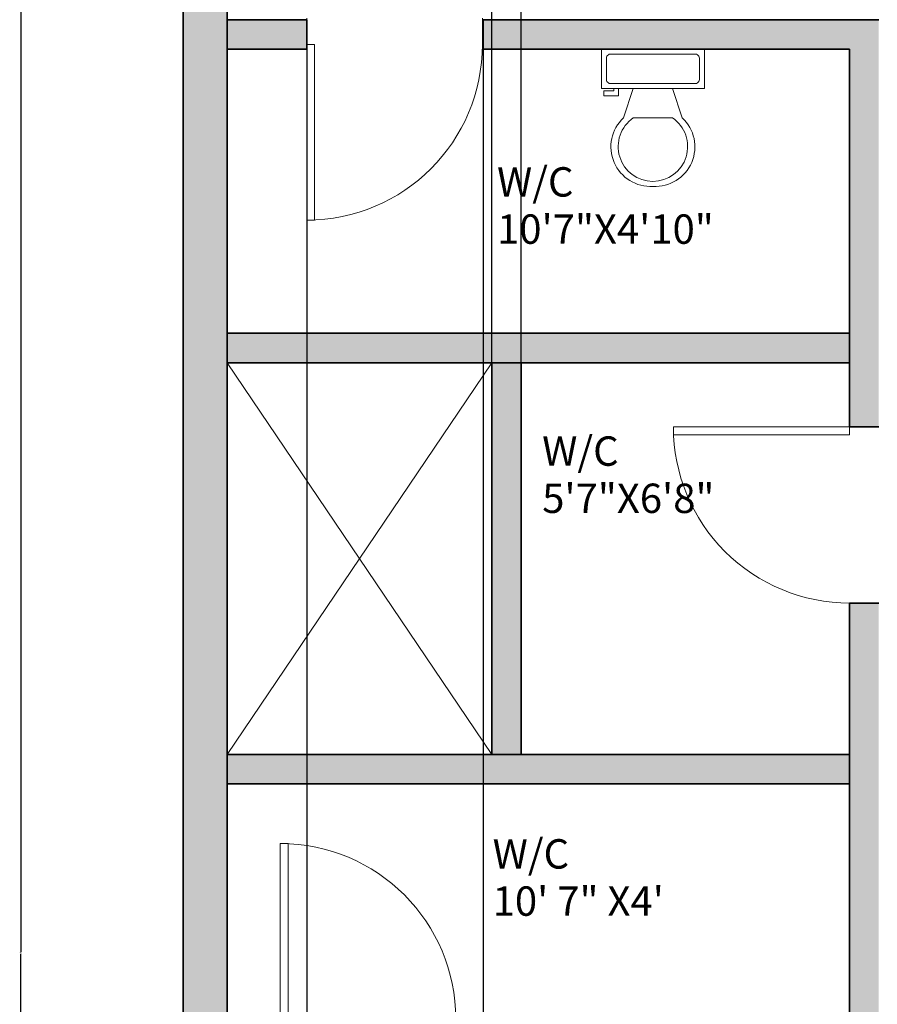
# Model space of a CAD drawing. Units: inches. Extents: x 2070 to 4408, y 1595 to 4269.
# Tile 9 of 20: x 2070 to 2245, y 1949 to 2150. Entities that reach past the tile are written whole.
import ezdxf

# ---------------------------------------------------------------- set-up
doc = ezdxf.new("R2010")
doc.units = ezdxf.units.IN
for name, color, linetype, lineweight in [('A-ANNO-DIMS', 2, 'Continuous', 18), ('A-AREA-IDEN', 7, 'Continuous', 18), ('A-DOOR', 4, 'Continuous', 18), ('A-FLOR-FIXT', 9, 'Continuous', 18), ('A-FLOR-OPEN', 8, 'Continuous', 13), ('A-WALL', 7, 'Continuous', 35)]:
    doc.layers.add(name, color=color, linetype=linetype, lineweight=lineweight)
doc.layers.add('A-WALL-PATT', color=18, linetype='Continuous', lineweight=13, true_color=0x000000)
doc.styles.get("Standard").update_dxf_attribs({"font": 'arial.ttf'})
doc.dimstyles.get("Standard").update_dxf_attribs({"dimtxt": 0.18, "dimasz": 0.18, "dimexe": 0.18, "dimexo": 0.0625, "dimgap": 0.09, "dimtad": 0, "dimtih": 1, "dimtoh": 1, "dimdec": 4, "dimzin": 0, "dimdsep": 46, "dimtxsty": 'Standard', "dimcen": 0.09, "dimadec": 0, "dimazin": 0, "dimtfac": 1, "dimtdec": 4, "dimtofl": 0, "dimtmove": 0, "dimatfit": 3, "dimfxl": 1, "dimtolj": 1, "dimtzin": 0, "dimarcsym": 0})

# ---------------------------------------------------------------- blocks, each defined once
blk = doc.blocks.new('*U3')
for p, q in [((0, 0), (0, 6)), ((40, 0), (40, 6))]:
    blk.add_line(p, q)
blk.add_lwpolyline([(0, 0), (0, -40), (1.75, -40), (1.75, 0)], close=True)
blk.add_arc((0, 0), 40, 270, 0)
blk = doc.blocks.new('*U4')
for p, q in [((0, 0), (0, -6)), ((40, 0), (40, -6))]:
    blk.add_line(p, q)
blk.add_lwpolyline([(0, 0), (0, 40), (1.75, 40), (1.75, 0)], close=True)
blk.add_arc((0, 0), 40, 0, 90)
blk = doc.blocks.new('*U11')
for p, q in [((241.3, -152.4), (241.3, -50.8)), ((-203.2, -215.9), (-203.2, -203.2)), ((-177.8, -203.2), (-177.8, -241.3)), ((-101.6, -203.2), (-152.4, -355.6)), ((101.6, -203.2), (152.4, -355.6)), ((-254, -215.9), (-203.2, -215.9)), ((-254, -241.3), (-254, -215.9)), ((-177.8, -241.3), (-254, -241.3)), ((101.6, -355.6), (-101.6, -355.6))]:
    blk.add_line(p, q)
blk.add_lwpolyline([(266.7, -203.2), (266.7, 0), (-266.7, 0), (-266.7, -203.2)], close=True)
for points in [[(-241.3, -50.8), (-241.3, -152.4)], [(215.9, -25.4), (-215.9, -25.4)], [(-215.9, -177.8), (215.9, -177.8)]]:
    blk.add_lwpolyline(points)
for centre, radius, start, end in [((-219.075, -47.625), 22.45064, 81.8699, 188.1301), ((219.075, -47.625), 22.45064, 351.8699, 98.1301), ((-219.075, -155.575), 22.45064, 171.869898, 278.1301), ((219.075, -155.575), 22.45064, 261.8699, 8.1301), ((-12.12088, -505.93752), 205.61935, 133.01722, 273.38), ((0.94996, -504.77674), 181.02486, 124.50543, 269.7), ((-0.94742, -504.77674), 181.02486, 270.3, 55.4946), ((12.12342, -505.93752), 205.61935, 266.62, 46.9828)]:
    blk.add_arc(centre, radius, start, end)
blk = doc.blocks.new('*D24')
at = {"layer": 'A-ANNO-DIMS', "color": 0, "lineweight": -2, "transparency": 16777216}
for p, q in [((2103.13, 2291.4), (2069.84, 2291.4)), ((2070.02, 2291.22), (2070.02, 1960.08)), ((2070.02, 1628.58), (2070.02, 1959.72)), ((2336.13, 1628.4), (2069.84, 1628.4))]:
    blk.add_line(p, q, dxfattribs=at)
at = {"layer": 'A-ANNO-DIMS', "color": 0, "transparency": 16777216}
for points in [[(2069.99, 2291.22), (2070.05, 2291.22), (2070.02, 2291.4)], [(2069.99, 1628.58), (2070.05, 1628.58), (2070.02, 1628.4)]]:
    blk.add_solid(points, dxfattribs=at)
at = {"layer": 'Defpoints', "color": 0, "transparency": 16777216}
for p in [(2070.02, 2291.4), (2103.2, 2291.4), (2336.2, 1628.4)]:
    blk.add_point(p, dxfattribs=at)
at = {"layer": 'A-ANNO-DIMS', "color": 0, "transparency": 16777216, "insert": (2070.02, 1959.9), "char_height": 0.18, "attachment_point": 5}
blk.add_mtext('\\A1;663', dxfattribs=at)
blk = doc.blocks.new('*D28')
at = {"layer": 'A-ANNO-DIMS', "color": 0, "lineweight": -2, "transparency": 16777216}
for p, q in [((2166.2, 2000.46), (2166.2, 2324.76)), ((2166.38, 2324.58), (2169.05, 2324.58)), ((2172.02, 2324.58), (2169.35, 2324.58)), ((2172.2, 2000.46), (2172.2, 2324.76))]:
    blk.add_line(p, q, dxfattribs=at)
at = {"layer": 'A-ANNO-DIMS', "color": 0, "transparency": 16777216}
for points in [[(2166.38, 2324.61), (2166.38, 2324.55), (2166.2, 2324.58)], [(2172.02, 2324.61), (2172.02, 2324.55), (2172.2, 2324.58)]]:
    blk.add_solid(points, dxfattribs=at)
at = {"layer": 'Defpoints', "color": 0, "transparency": 16777216}
for p in [(2172.2, 2324.58), (2166.2, 2000.4), (2172.2, 2000.4)]:
    blk.add_point(p, dxfattribs=at)
at = {"layer": 'A-ANNO-DIMS', "color": 0, "transparency": 16777216, "insert": (2169.2, 2324.58), "char_height": 0.18, "attachment_point": 5}
blk.add_mtext('\\A1;6', dxfattribs=at)
blk = doc.blocks.new('*D29')
at = {"layer": 'A-ANNO-DIMS', "color": 0, "lineweight": -2, "transparency": 16777216}
for p, q in [((2128.44, 2150.34), (2128.44, 1595.04)), ((2164.44, 2150.34), (2164.44, 1595.04)), ((2128.62, 1595.22), (2146.22, 1595.22)), ((2164.26, 1595.22), (2146.65, 1595.22))]:
    blk.add_line(p, q, dxfattribs=at)
at = {"layer": 'A-ANNO-DIMS', "color": 0, "transparency": 16777216}
for points in [[(2128.62, 1595.25), (2128.62, 1595.19), (2128.44, 1595.22)], [(2164.26, 1595.25), (2164.26, 1595.19), (2164.44, 1595.22)]]:
    blk.add_solid(points, dxfattribs=at)
at = {"layer": 'Defpoints', "color": 0, "transparency": 16777216}
for p in [(2128.44, 2150.4), (2164.44, 2150.4), (2164.44, 1595.22)]:
    blk.add_point(p, dxfattribs=at)
at = {"layer": 'A-ANNO-DIMS', "color": 0, "transparency": 16777216, "insert": (2146.44, 1595.22), "char_height": 0.18, "attachment_point": 5}
blk.add_mtext('\\A1;36', dxfattribs=at)
blk = doc.blocks.new('*D31')
at = {"layer": 'A-ANNO-DIMS', "color": 0, "lineweight": -2, "transparency": 16777216}
for p, q in [((2112.2, 2000.46), (2112.2, 2324.76)), ((2112.38, 2324.58), (2138.98, 2324.58)), ((2166.02, 2324.58), (2139.41, 2324.58)), ((2166.2, 2000.46), (2166.2, 2324.76))]:
    blk.add_line(p, q, dxfattribs=at)
at = {"layer": 'A-ANNO-DIMS', "color": 0, "transparency": 16777216}
for points in [[(2112.38, 2324.61), (2112.38, 2324.55), (2112.2, 2324.58)], [(2166.02, 2324.61), (2166.02, 2324.55), (2166.2, 2324.58)]]:
    blk.add_solid(points, dxfattribs=at)
at = {"layer": 'Defpoints', "color": 0, "transparency": 16777216}
for p in [(2166.2, 2324.58), (2112.2, 2000.4), (2166.2, 2000.4)]:
    blk.add_point(p, dxfattribs=at)
at = {"layer": 'A-ANNO-DIMS', "color": 0, "transparency": 16777216, "insert": (2139.2, 2324.58), "char_height": 0.18, "attachment_point": 5}
blk.add_mtext('\\A1;54', dxfattribs=at)

msp = doc.modelspace()

# ---------------------------------------------------------------- hatches: boundary and pattern name
at = {"layer": 'A-WALL-PATT'}
h = msp.add_hatch(color=256, dxfattribs=at)
h.dxf.hatch_style = 1
h.paths.add_polyline_path([(2346.196, 2218.3995), (2346.196, 2282.3995), (2340.196, 2282.3995), (2340.196, 2212.3995), (2345.5866, 2212.3995), (2346.196, 2212.3995)], flags=0)
h.paths.add_polyline_path([(2245.196, 2282.3995), (2239.196, 2282.3995), (2239.196, 2186.3995), (2244.5866, 2186.3995), (2245.196, 2186.3995)], flags=0)
h.paths.add_polyline_path([(2340.196, 2230.6455), (2245.196, 2230.6455), (2245.196, 2224.6455), (2340.196, 2224.6455)], flags=0)
h.paths.add_polyline_path([(2245.196, 2150.3995), (2239.196, 2150.3995), (2164.4362, 2150.3995), (2164.4362, 2144.3995), (2239.196, 2144.3995), (2239.196, 2086.3995), (2239.196, 2067.2711), (2244.5866, 2067.2711), (2245.196, 2067.2711), (2245.196, 2144.3995)], flags=0)
h.paths.add_polyline_path([(2346.196, 2176.3995), (2340.196, 2176.3995), (2340.196, 2086.3995), (2346.196, 2086.3995), (2346.196, 2125.318)], flags=0)
h.paths.add_polyline_path([(2446.196, 2086.3995), (2346.196, 2086.3995), (2340.196, 2086.3995), (2340.196, 2080.3995), (2446.196, 2080.3995)], flags=0)
h.paths.add_polyline_path([(2455.196, 2291.3995), (2103.196, 2291.3995), (2103.196, 1699.3995), (2336.196, 1699.3995), (2336.196, 1628.3995), (2345.196, 1628.3995), (2446.196, 1628.3995), (2454.8846, 1628.3995), (2454.8846, 1699.3995)])
h.paths.add_polyline_path([(2446.196, 2282.3995), (2446.196, 2218.3995), (2446.196, 2212.3995), (2446.196, 2086.3995), (2446.196, 2080.3995), (2446.196, 1708.3995), (2446.196, 1637.3995), (2345.196, 1637.3995), (2345.196, 1699.3995), (2345.196, 1708.3995), (2336.196, 1708.3995), (2112.196, 1708.3995), (2112.196, 2282.3995), (2239.196, 2282.3995), (2245.196, 2282.3995), (2356.196, 2282.3995)], flags=16)
h.paths.add_polyline_path([(2245.196, 2150.3995), (2245.196, 2144.3995), (2245.196, 2067.2711), (2244.5866, 2067.2711), (2239.196, 2067.2711), (2239.196, 2065.6988), (2203.2929, 2065.6988, 0.40145271), (2239.196, 2031.3337), (2244.5866, 2031.3337), (2245.196, 2031.2711), (2245.196, 1924.1525), (2239.196, 1924.1525), (2239.196, 1922.5803), (2203.2929, 1922.5803, 0.40145271), (2239.196, 1888.2151), (2244.5866, 1888.2151), (2245.196, 1888.1525), (2245.196, 1748.3995), (2339.196, 1748.4621, -0.40145271), (2303.2929, 1782.8272), (2303.2585, 1782.8272), (2303.2585, 1784.3995), (2339.196, 1784.3995), (2339.196, 1877.2067), (2291.196, 1877.2067), (2291.196, 1883.2067), (2291.196, 1946.3995), (2291.196, 1952.3995), (2291.196, 2086.3995), (2297.196, 2086.3995), (2302.196, 2086.3995), (2302.196, 2081.0259), (2303.7633, 2081.0259), (2303.7633, 2080.3995), (2338.0148, 2080.3995, 0.00437129), (2338.0203, 2081.0259), (2338.0203, 2086.3995), (2340.196, 2086.3995), (2340.196, 2176.4621), (2345.5866, 2176.4621, 0.40145271), (2381.4896, 2210.8272), (2345.5866, 2210.8272), (2345.5866, 2212.3995), (2340.196, 2212.3995), (2340.196, 2224.6455), (2245.196, 2224.6455), (2245.196, 2186.3995), (2244.5866, 2186.3995), (2239.196, 2186.3995), (2239.196, 2184.8272), (2203.2929, 2184.8272, 0.40145271), (2239.196, 2150.4621), (2244.5866, 2150.4621)], flags=0)
h.paths.add_polyline_path([(2346.196, 2282.3995), (2346.196, 2218.3995), (2377.1813, 2218.3995), (2377.1813, 2212.3995), (2346.196, 2212.3995), (2345.5866, 2212.3995), (2340.196, 2212.3995), (2340.196, 2224.6455), (2245.196, 2224.6455), (2245.196, 2230.6455), (2245.196, 2282.3995), (2292.696, 2256.5225), (2340.196, 2282.3995)], flags=0)
h.paths.add_polyline_path([(2346.196, 2086.3995), (2340.196, 2086.3995), (2340.196, 2080.3995), (2446.196, 2080.3995), (2431.196, 2016.3995), (2446.196, 1952.3995), (2412.196, 1952.3995), (2412.196, 2080.3995), (2340.196, 2080.3995), (2340.196, 2086.3995), (2340.196, 2176.3995), (2346.196, 2176.3995), (2346.196, 2125.318)], flags=0)
h.paths.add_polyline_path([(2186.508, 2270.0471, -0.03755288), (2186.9712, 2269.8581), (2186.9164, 2270.112, -0.02759121)], flags=0)
h.paths.add_polyline_path([(2183.955, 2273.7766, 1), (2188.2945, 2273.7766, 1)], flags=0)
h.paths.add_polyline_path([(2142.5261, 2274.6158, -0.03707541), (2142.5672, 2275.1696), (2142.5672, 2276.826), (2119.8759, 2276.826), (2119.8759, 2263.0962), (2140.4332, 2263.0962), (2142.5672, 2263.0962), (2142.5672, 2274.0621, -0.03707541)], flags=0)
h.paths.add_polyline_path([(2209.8974, 2263.0962), (2209.8974, 2262.2079), (2190.8042, 2262.2079), (2190.8042, 2263.0962)], flags=0)
h.paths.add_polyline_path([(2210.6382, 2276.1833), (2210.6382, 2263.9844), (2190.2185, 2263.9844), (2190.2185, 2276.1833)], flags=0)
h.paths.add_polyline_path([(2188.4362, 2273.7766, -1), (2183.8133, 2273.7766, -1)], flags=0)
h.paths.add_polyline_path([(2245.196, 2150.3995), (2245.196, 2144.3995), (2245.196, 2067.2711), (2239.196, 2067.2711), (2239.196, 2080.3995), (2172.196, 2080.3995), (2172.196, 2000.3995), (2239.196, 2000.3995), (2239.196, 1940.3995), (2159.0187, 1940.3995), (2123.0187, 1940.3995), (2112.196, 1940.3995), (2112.196, 1946.3995), (2123.0187, 1946.3995), (2123.0187, 1982.2238), (2124.586, 1982.2238), (2124.586, 1982.1895, -0.40145271), (2158.8429, 1946.3995), (2159.0187, 1946.3995), (2239.196, 1946.3995), (2239.196, 1994.3995), (2112.196, 1994.3995), (2112.196, 2000.3995), (2139.196, 2040.3995), (2112.196, 2080.3995), (2112.196, 2086.3995), (2239.196, 2086.3995), (2239.196, 2144.3995), (2209.5809, 2144.3995), (2209.5809, 2136.3995), (2203.0809, 2136.3995), (2205.0809, 2130.3996, -0.70257121), (2199.081, 2116.3995, -0.70256205), (2193.0809, 2130.3994), (2195.0809, 2136.3995), (2192.0809, 2136.3995), (2192.0809, 2134.8995), (2189.0809, 2134.8995), (2189.0809, 2135.8995), (2191.0809, 2135.8995), (2191.0809, 2136.3995), (2188.5809, 2136.3995), (2188.5809, 2144.3995), (2164.2481, 2144.3995, -0.39385849), (2130.0035, 2109.5491), (2130.0035, 2109.5147), (2128.4362, 2109.5147), (2128.4362, 2144.3995), (2112.196, 2144.3995), (2112.196, 2150.3995), (2128.4362, 2150.3995), (2128.4362, 2150.7127), (2164.4362, 2150.7127), (2164.4362, 2150.3995), (2239.196, 2150.3995)], flags=0)
h.paths.add_polyline_path([(2188.2075, 2266.8735), (2188.2075, 2211.8632, -0.41421356), (2185.4833, 2209.1391), (2146.7995, 2209.1391, -0.41421356), (2144.0754, 2211.8632), (2144.0754, 2266.8735, -0.41421356), (2146.7995, 2269.5976), (2185.4833, 2269.5976, -0.41421356)], flags=0)
h.paths.add_polyline_path([(2185.0844, 2273.7766, -1), (2187.1651, 2273.7766, -1)], flags=0)
h.paths.add_polyline_path([(2182.0486, 2259.2932), (2168.0953, 2259.2932), (2168.0953, 2260.8424), (2163.7261, 2260.8424), (2163.7261, 2259.2932), (2149.7727, 2259.2932), (2149.7727, 2266.3352), (2163.7261, 2266.3352), (2163.7261, 2261.9839), (2168.0953, 2261.9839), (2168.0953, 2266.3352), (2182.0486, 2266.3352)], flags=0)
h.paths.add_polyline_path([(2148.2585, 2250.2051), (2153.0615, 2241.8861, 0.39807048)], flags=0)
h.paths.add_polyline_path([(2162.7572, 2247.2885), (2153.1461, 2241.7396), (2148.1083, 2250.4653), (2157.7194, 2256.0142)], flags=0)
h.paths.add_polyline_path([(2162.6726, 2247.4351, -0.39286196), (2157.8415, 2255.6313), (2157.6431, 2255.6313), (2157.8696, 2255.7541)], flags=0)
h.paths.add_polyline_path([(2164.2604, 2145.339), (2164.4362, 2144.3995), (2164.4362, 2150.3995), (2164.2604, 2150.7127)], flags=0)
h.paths.add_polyline_path([(2208.5809, 2142.6495), (2208.5809, 2138.3995, -0.41421356), (2207.8309, 2137.3995), (2190.5809, 2137.3995, -0.41421356), (2189.5809, 2138.1495), (2189.5809, 2142.3995, -0.41421356), (2190.3309, 2143.3995), (2207.5809, 2143.3995, -0.41421356)], flags=0)
h.paths.add_polyline_path([(2147.957, 2229.9119), (2154.7494, 2223.1195, 0.39807048)], flags=0)
h.paths.add_polyline_path([(2162.7165, 2230.8473), (2154.8691, 2222.9998), (2147.7446, 2230.1244), (2155.592, 2237.9718)], flags=0)
h.paths.add_polyline_path([(2162.5969, 2230.9669, -0.39807048), (2155.8044, 2237.7594)], flags=0)
h.paths.add_polyline_path([(2391.8776, 2049.9192), (2408.5766, 2049.9192), (2408.5766, 2033.2202), (2408.5766, 1983.123), (2408.5766, 1966.4239), (2391.8776, 1966.4239), (2391.8776, 1983.123), (2341.7804, 1983.123), (2341.7804, 2033.2202), (2391.8776, 2033.2202)], flags=0)
h.paths.add_polyline_path([(2144.1055, 2274.6158, 1), (2148.445, 2274.6158, 1)], flags=0)
h.paths.add_polyline_path([(2148.5867, 2274.6158, -1), (2143.9638, 2274.6158, -1)], flags=0)
h.paths.add_polyline_path([(2145.2349, 2274.6158, -1), (2147.3156, 2274.6158, -1)], flags=0)
edge = h.paths.add_edge_path(flags=0)
edge.add_ellipse((2400.5951, 2040.9436), major_axis=(-4.5109, 0), ratio=0.97544784, start_angle=180, end_angle=270, ccw=False)
edge.add_ellipse((2400.5951, 2040.9436), major_axis=(-4.5109, 0), ratio=0.97544784, start_angle=90, end_angle=180, ccw=False)
edge.add_ellipse((2400.5951, 2040.9436), major_axis=(-4.5109, 0), ratio=0.97544784, start_angle=0, end_angle=90, ccw=False)
edge.add_ellipse((2400.5951, 2040.9436), major_axis=(-4.5109, 0), ratio=0.97544784, start_angle=270, end_angle=360, ccw=False)
h.paths.add_polyline_path([(2199.0809, 2117.3995, -0.73452973), (2195.0809, 2130.3995), (2203.081, 2130.3995, -0.73453329)], flags=0)
h.paths.add_polyline_path([(2141.9147, 2276.0353), (2141.9147, 2263.9844), (2120.4685, 2263.9844), (2120.4685, 2276.0353)], flags=0)
h.paths.add_polyline_path([(2138.4481, 2273.4072), (2138.4481, 2266.7226), (2133.2801, 2266.7226), (2133.2801, 2273.4072)], flags=0)
h.paths.add_polyline_path([(2137.9691, 2272.9175), (2137.9691, 2272.204), (2135.4229, 2272.204), (2135.4229, 2271.6329), (2135.3221, 2270.1051), (2135.3221, 2269.0265), (2135.4229, 2268.6811), (2135.4229, 2267.2011), (2133.7212, 2267.2011), (2133.7212, 2268.6811), (2133.7983, 2269.9587), (2133.7983, 2271.2758), (2133.7212, 2271.6329), (2133.7212, 2273.0065), (2135.717, 2273.0065), (2135.717, 2272.9175)], flags=0)
h.paths.add_polyline_path([(2137.9215, 2271.8264), (2137.9215, 2271.3786), (2137.5182, 2271.3786), (2136.9355, 2271.3786), (2136.3529, 2271.3786), (2135.7703, 2271.3786), (2135.7703, 2271.8264), (2136.1736, 2271.8264), (2136.7562, 2271.8264), (2137.3389, 2271.8264)], flags=0)
h.paths.add_polyline_path([(2137.9215, 2271.692), (2137.5182, 2271.692), (2136.9355, 2271.513), (2137.3389, 2271.513)], flags=0)
h.paths.add_polyline_path([(2136.3529, 2271.692), (2135.7703, 2271.513), (2136.1736, 2271.513), (2136.7562, 2271.692)], flags=0)
h.paths.add_polyline_path([(2137.9215, 2271.513), (2137.5182, 2271.513), (2136.7562, 2271.747), (2136.7562, 2271.692), (2137.3389, 2271.692)], flags=0)
h.paths.add_polyline_path([(2137.8207, 2270.4664), (2137.8207, 2270.0971), (2137.8207, 2269.627), (2137.8207, 2269.1569), (2137.8207, 2268.6868), (2137.3837, 2268.6868), (2136.6442, 2268.6868), (2135.9271, 2268.6868), (2135.9271, 2269.0562), (2135.9271, 2269.5263), (2135.9271, 2269.9963), (2135.9271, 2270.4664), (2136.3641, 2270.4664), (2137.0812, 2270.4664)], flags=0)
h.paths.add_polyline_path([(2137.3837, 2269.627), (2137.8207, 2269.627), (2137.8207, 2269.5263), (2137.3837, 2269.5263), (2137.3837, 2269.1569), (2137.8207, 2269.1569), (2137.3837, 2269.0562), (2137.3837, 2268.6868), (2137.0812, 2268.6868), (2137.0812, 2269.0562), (2136.6442, 2269.0562), (2136.6442, 2268.6868), (2136.3641, 2268.6868), (2136.3641, 2269.0562), (2135.9271, 2269.0562), (2135.9271, 2269.1569), (2136.3641, 2269.1569), (2136.3641, 2269.5263), (2135.9271, 2269.5263), (2135.9271, 2269.627), (2136.3641, 2269.627), (2136.3641, 2269.9963), (2135.9271, 2269.9963), (2136.3641, 2270.0971), (2136.3641, 2270.4664), (2136.6442, 2270.4664), (2136.6442, 2270.0971), (2137.0812, 2270.0971), (2137.0812, 2270.4664), (2137.3837, 2270.4664), (2137.3837, 2270.0971), (2137.8207, 2270.0971), (2137.3837, 2269.9963)], flags=0)
h.paths.add_polyline_path([(2137.5182, 2271.8264), (2137.5182, 2271.692), (2137.3389, 2271.3786), (2137.3389, 2271.513)], flags=0)
h.paths.add_polyline_path([(2137.8179, 2267.8138), (2137.8179, 2267.6879), (2137.1876, 2267.6879), (2136.4733, 2267.6879), (2135.759, 2267.6879), (2135.759, 2267.8138), (2136.3893, 2267.8138), (2137.1036, 2267.8138)], flags=0)
h.paths.add_polyline_path([(2137.0812, 2269.9963), (2137.0812, 2269.627), (2137.0812, 2269.1569), (2136.6442, 2269.1569), (2136.6442, 2269.5263), (2136.6442, 2269.9963)], flags=0)
h.paths.add_polyline_path([(2136.3529, 2271.8264), (2136.3529, 2271.692), (2136.1736, 2271.3786), (2136.1736, 2271.513)], flags=0)
h.paths.add_polyline_path([(2136.4733, 2267.8138), (2136.4733, 2267.6879), (2136.3893, 2267.6879), (2136.3893, 2267.8138)], flags=0)
h.paths.add_polyline_path([(2407.9087, 2032.5522), (2407.9087, 1983.7909), (2359.81, 1983.7909, -0.00912788), (2359.0575, 1983.7909), (2342.4483, 1983.7909), (2342.4483, 2032.5522)], flags=0)
h.paths.add_polyline_path([(2389.1838, 2023.1358), (2353.7856, 2023.1358), (2353.7856, 1985.4867, -0.09210376), (2350.2788, 1988.655), (2350.2788, 2026.6426), (2389.1838, 2026.6426)], flags=0)
h.paths.add_polyline_path([(2352.6166, 2024.3048), (2351.4477, 2024.3048), (2351.4477, 2025.4737), (2352.6166, 2025.4737)], flags=0)
h.paths.add_polyline_path([(2399.6319, 2026.7589), (2404.3661, 2026.7589, -0.41421356), (2407.0379, 2024.087), (2407.0379, 2013.4908, -0.41421356), (2404.3661, 2010.819), (2399.6319, 2010.819, -0.41421356), (2396.96, 2013.4908), (2396.96, 2024.087, -0.41421356)], flags=0)
h.paths.add_polyline_path([(2399.6319, 2026.0909), (2404.3661, 2026.0909, -0.41421356), (2406.37, 2024.087), (2406.37, 2013.4908, -0.41421356), (2404.3661, 2011.487), (2399.6319, 2011.487, -0.41421356), (2397.628, 2013.4908), (2397.628, 2024.087, -0.41421356)], flags=0)
h.paths.add_polyline_path([(2399.6319, 2002.3217), (2404.3661, 2002.3217, -0.41421356), (2407.0379, 1999.6498), (2407.0379, 1989.0536, -0.41421356), (2404.3661, 1986.3818), (2399.6319, 1986.3818, -0.41421356), (2396.96, 1989.0536), (2396.96, 1999.6498, -0.41421356)], flags=0)
h.paths.add_polyline_path([(2399.6319, 2001.6537), (2404.3661, 2001.6537, -0.41421356), (2406.37, 1999.6498), (2406.37, 1989.0536, -0.41421356), (2404.3661, 1987.0497), (2399.6319, 1987.0497, -0.41421356), (2397.628, 1989.0536), (2397.628, 1999.6498, -0.41421356)], flags=0)
edge = h.paths.add_edge_path(flags=0)
edge.add_ellipse((2400.5951, 1975.3996), major_axis=(-4.5109, 0), ratio=0.97544784, start_angle=-180, end_angle=-90, ccw=False)
edge.add_ellipse((2400.5951, 1975.3996), major_axis=(-4.5109, 0), ratio=0.97544784, start_angle=90, end_angle=180, ccw=False)
edge.add_ellipse((2400.5951, 1975.3996), major_axis=(-4.5109, 0), ratio=0.97544784, start_angle=0, end_angle=90, ccw=False)
edge.add_ellipse((2400.5951, 1975.3996), major_axis=(-4.5109, 0), ratio=0.97544784, start_angle=-90, end_angle=0, ccw=False)
h.paths.add_polyline_path([(2345.196, 1910.3995), (2366.4386, 1910.3995), (2366.4386, 1925.4555), (2392.3856, 1925.4555), (2392.3856, 1933.5025), (2400.1399, 1925.4555), (2392.3856, 1919.8795), (2392.3856, 1925.4555), (2366.4386, 1925.4555), (2366.4386, 1910.3995), (2381.196, 1910.3995), (2405.196, 1910.3995), (2405.196, 1898.3995), (2446.196, 1898.3995), (2446.196, 1886.3995), (2405.196, 1886.3995), (2405.196, 1874.3995), (2446.196, 1874.3995), (2446.196, 1862.3995), (2405.196, 1862.3995), (2405.196, 1850.3995), (2446.196, 1850.3995), (2446.196, 1838.3995), (2405.196, 1838.3995), (2405.196, 1826.3995), (2446.196, 1826.3995), (2446.196, 1814.3995), (2405.196, 1814.3995), (2405.196, 1802.3995), (2446.196, 1802.3995), (2446.196, 1798.3995), (2446.196, 1792.3995), (2405.196, 1792.3995), (2405.196, 1910.3995), (2381.196, 1910.3995), (2381.196, 1792.3995), (2345.196, 1792.3995)], flags=0)
h.paths.add_polyline_path([(2333.0944, 1863.3993, -0.41421356), (2334.7225, 1861.7712), (2334.7225, 1859.329), (2335.2653, 1859.329, -0.41421356), (2337.4361, 1857.1582), (2337.4361, 1843.862, -0.41421356), (2335.2653, 1841.6911, -0.41421356), (2337.4361, 1839.5203), (2337.4361, 1827.5808, -0.41421356), (2335.2653, 1825.41, -0.41421356), (2337.4361, 1823.2392), (2337.4361, 1808.5862, -0.41421356), (2335.2653, 1806.4153), (2334.7225, 1806.4153), (2334.7225, 1803.9732, -0.41421356), (2333.0944, 1802.3451), (2317.356, 1802.3451), (2317.0846, 1802.3451, -0.41421356), (2315.7279, 1803.7018), (2315.7279, 1803.8646), (2313.8284, 1803.8646, -0.41421356), (2311.6576, 1806.0354), (2311.6576, 1823.2015, -0.39597602), (2313.6834, 1825.3765, -0.43384798), (2311.6576, 1827.2718), (2311.6576, 1839.761, -0.41421356), (2313.5571, 1841.6604), (2313.8284, 1841.6604), (2333.8159, 1841.6604, -0.04213623), (2334.1798, 1841.6911, -0.41421356), (2332.009, 1843.862), (2332.009, 1857.1582, -0.41421356), (2334.1798, 1859.329), (2317.356, 1859.329), (2317.0846, 1859.329, -0.41421356), (2315.7279, 1860.6858), (2315.7279, 1862.0426, -0.41421356), (2317.0846, 1863.3993), (2317.356, 1863.3993)], flags=0)
h.paths.add_polyline_path([(2208.8475, 1848.9818), (2208.8475, 1840.9741, -0.41421356), (2207.0458, 1839.1724), (2206.5453, 1839.1721), (2206.5453, 1838.7218, -0.40985861), (2204.7704, 1836.9203), (2183.7501, 1836.9203, -0.41858196), (2181.9216, 1838.7218), (2181.9216, 1839.1721), (2181.421, 1839.1724, -0.41421356), (2179.6193, 1840.9741), (2179.6193, 1848.6817, -0.44064415), (2185.1126, 1854.9874), (2203.3852, 1854.9874, -0.45707961)], flags=0)
h.paths.add_polyline_path([(2204.243, 1848.4815), (2204.243, 1848.4815, 0.41725335), (2202.2204, 1850.4833), (2186.2049, 1850.4833, 0.4111805), (2184.2237, 1848.4815), (2184.2237, 1848.4815, -0.4111807), (2186.2049, 1850.4833), (2202.2204, 1850.4833, -0.41725315)], flags=0)
h.paths.add_polyline_path([(2234.7177, 1830.228), (2234.7176, 1781.6047, -0.41421356), (2233.4381, 1780.3252), (2218.6064, 1780.3252, -0.41421356), (2217.8387, 1781.0929), (2217.8387, 1783.3961, -0.41421356), (2218.6064, 1784.1639), (2218.6065, 1796.9595, -0.41421356), (2219.886, 1798.239, -0.41421356), (2218.6065, 1799.5186), (2218.6065, 1812.3142, -0.41421356), (2219.8861, 1813.5938, -0.41421356), (2218.6065, 1814.8733), (2218.6065, 1827.6689, -0.41421356), (2217.8388, 1828.4367), (2217.8388, 1830.7399, -0.41421356), (2218.6065, 1831.5076), (2233.4382, 1831.5076, -0.41421356)], flags=0)
h.paths.add_polyline_path([(2230.6344, 1827.6689, -0.41421356), (2231.4021, 1826.9012), (2231.4021, 1784.9316, -0.41421356), (2230.6343, 1784.1639), (2221.1853, 1784.1639), (2221.1853, 1827.6689)], flags=0)
h.paths.add_polyline_path([(2222.7208, 1798.239), (2221.6971, 1798.239), (2221.6971, 1813.5938), (2222.7208, 1813.5938)], flags=0)
h.paths.add_polyline_path([(2206.5453, 1773.935), (2206.5453, 1773.4848), (2206.9457, 1773.4848), (2207.0458, 1773.4845, -0.41421356), (2208.8475, 1771.6827), (2208.8475, 1763.675, -0.44222432), (2203.6505, 1757.6695), (2185.3851, 1757.6695, -0.45508402), (2179.6193, 1763.9752), (2179.6193, 1771.6827, -0.41421356), (2181.421, 1773.4845), (2181.421, 1773.4848), (2181.9216, 1773.4848), (2181.9216, 1773.935, -0.40985861), (2183.6965, 1775.7366), (2204.7167, 1775.7366, -0.41858196)], flags=0)
h.paths.add_polyline_path([(2202.2619, 1762.1736), (2186.2464, 1762.1736, -0.41725315), (2184.2237, 1764.1754), (2184.2237, 1764.1754, 0.41725335), (2186.2464, 1762.1736), (2202.2619, 1762.1736, 0.4111805), (2204.243, 1764.1754), (2204.243, 1764.1754, -0.4111807)], flags=0)
h.paths.add_polyline_path([(2313.0034, 1713.1906), (2312.997, 1713.1697), (2313.0123, 1713.1612)], flags=0)
h.paths.add_polyline_path([(2305.7314, 1721.0488), (2305.6257, 1721.1994), (2305.4853, 1721.084)], flags=0)
h.paths.add_polyline_path([(2307.5562, 1726.1427), (2307.6186, 1726.1026), (2307.5737, 1726.0477), (2308.5692, 1720.6434), (2310.5345, 1721.2985), (2310.5721, 1721.411), (2310.6958, 1721.3523), (2313.8453, 1722.4021), (2314.9351, 1723.8033), (2314.9294, 1723.9165), (2315.0028, 1723.8903), (2313.874, 1722.4389), (2313.8697, 1722.4102), (2308.5692, 1720.6434), (2308.9864, 1720.122), (2309.0665, 1720.0971), (2309.053, 1720.0387), (2310.9235, 1717.7005), (2311.4182, 1717.6259), (2311.2918, 1717.2402), (2312.0655, 1716.2731), (2312.1081, 1716.2606), (2312.0969, 1716.2339), (2308.5692, 1720.6434), (2305.2249, 1717.745), (2305.232, 1717.704), (2305.1665, 1717.6944), (2308.5692, 1720.6434)], flags=0)
h.paths.add_polyline_path([(2288.2072, 1714.3431), (2288.2008, 1714.3222), (2288.216, 1714.3137)], flags=0)
h.paths.add_polyline_path([(2280.9352, 1722.2013), (2280.8295, 1722.3519), (2280.689, 1722.2365)], flags=0)
h.paths.add_polyline_path([(2282.76, 1727.2952), (2282.8224, 1727.2551), (2282.7775, 1727.2002), (2283.773, 1721.7959), (2285.7383, 1722.451), (2285.7759, 1722.5635), (2285.8995, 1722.5048), (2289.0491, 1723.5546), (2290.1389, 1724.9558), (2290.1332, 1725.069), (2290.2065, 1725.0428), (2289.0777, 1723.5915), (2289.0735, 1723.5628), (2283.773, 1721.7959), (2284.1901, 1721.2745), (2284.2703, 1721.2496), (2284.2567, 1721.1913), (2286.1273, 1718.8531), (2286.622, 1718.7785), (2286.4956, 1718.3927), (2287.2692, 1717.4256), (2287.3119, 1717.4131), (2287.3006, 1717.3864), (2283.773, 1721.7959), (2280.4286, 1718.8975), (2280.4357, 1718.8565), (2280.3703, 1718.8469), (2283.773, 1721.7959)], flags=0)
h.paths.add_polyline_path([(2302.0672, 1721.8694), (2301.8205, 1721.8572), (2301.7578, 1722.1787), (2299.415, 1724.5215), (2299.103, 1724.4694), (2299.0662, 1724.8703)], flags=0)
h.paths.add_polyline_path([(2264.5643, 1715.4956), (2264.5579, 1715.4747), (2264.5731, 1715.4662)], flags=0)
h.paths.add_polyline_path([(2257.2923, 1723.3538), (2257.1865, 1723.5044), (2257.0461, 1723.389)], flags=0)
h.paths.add_polyline_path([(2259.117, 1728.4477), (2259.1795, 1728.4077), (2259.1345, 1728.3527), (2260.13, 1722.9484), (2262.0954, 1723.6036), (2262.133, 1723.716), (2262.2566, 1723.6573), (2265.4061, 1724.7071), (2266.4959, 1726.1083), (2266.4902, 1726.2215), (2266.5636, 1726.1953), (2265.4348, 1724.744), (2265.4305, 1724.7153), (2260.13, 1722.9484), (2260.5472, 1722.427), (2260.6273, 1722.4022), (2260.6138, 1722.3438), (2262.4843, 1720.0056), (2262.979, 1719.931), (2262.8526, 1719.5452), (2263.6263, 1718.5781), (2263.6689, 1718.5656), (2263.6577, 1718.5389), (2260.13, 1722.9484), (2256.7857, 1720.05), (2256.7928, 1720.009), (2256.7273, 1719.9994), (2260.13, 1722.9484)], flags=0)
h.paths.add_polyline_path([(2277.2709, 1723.0219), (2277.0243, 1723.0097), (2276.9616, 1723.3312), (2274.6187, 1725.6741), (2274.3067, 1725.6219), (2274.27, 1726.0228)], flags=0)
h.paths.add_polyline_path([(2253.628, 1724.1744), (2253.3814, 1724.1622), (2253.3186, 1724.4838), (2250.9758, 1726.8266), (2250.6638, 1726.7744), (2250.627, 1727.1753)], flags=0)
h.paths.add_polyline_path([(2161.9194, 1715.4956), (2161.913, 1715.4747), (2161.9282, 1715.4662)], flags=0)
h.paths.add_polyline_path([(2154.6474, 1723.3538), (2154.5416, 1723.5044), (2154.4012, 1723.389)], flags=0)
h.paths.add_polyline_path([(2162.7899, 1724.744), (2162.7856, 1724.7153), (2157.4851, 1722.9484), (2157.9023, 1722.427), (2157.9824, 1722.4022), (2157.9689, 1722.3438), (2159.8394, 1720.0056), (2160.3341, 1719.931), (2160.2078, 1719.5452), (2160.9814, 1718.5781), (2161.024, 1718.5656), (2161.0128, 1718.5389), (2157.4851, 1722.9484), (2154.1408, 1720.05), (2154.1479, 1720.009), (2154.0824, 1719.9994), (2157.4851, 1722.9484), (2156.4721, 1728.4477), (2156.5346, 1728.4077), (2156.4896, 1728.3527), (2157.4851, 1722.9484), (2159.4505, 1723.6036), (2159.4881, 1723.716), (2159.6117, 1723.6573), (2162.7612, 1724.7071), (2163.851, 1726.1083), (2163.8453, 1726.2215), (2163.9187, 1726.1953)], flags=0)
h.paths.add_polyline_path([(2150.9831, 1724.1744), (2150.7365, 1724.1622), (2150.6738, 1724.4838), (2148.3309, 1726.8266), (2148.0189, 1726.7744), (2147.9822, 1727.1753)], flags=0)
h.paths.add_polyline_path([(2132.5099, 1716.6482), (2132.5035, 1716.6272), (2132.5187, 1716.6187)], flags=0)
h.paths.add_polyline_path([(2125.2379, 1724.5064), (2125.1322, 1724.6569), (2124.9917, 1724.5415)], flags=0)
h.paths.add_polyline_path([(2133.3804, 1725.8965), (2133.3762, 1725.8678), (2128.0757, 1724.101), (2128.4928, 1723.5795), (2128.5729, 1723.5547), (2128.5594, 1723.4963), (2130.43, 1721.1581), (2130.9246, 1721.0835), (2130.7983, 1720.6977), (2131.5719, 1719.7306), (2131.6146, 1719.7181), (2131.6033, 1719.6914), (2128.0757, 1724.101), (2124.7313, 1721.2025), (2124.7384, 1721.1615), (2124.6729, 1721.1519), (2128.0757, 1724.101), (2127.0626, 1729.6002), (2127.1251, 1729.5602), (2127.0801, 1729.5052), (2128.0757, 1724.101), (2130.041, 1724.7561), (2130.0786, 1724.8685), (2130.2022, 1724.8098), (2133.3517, 1725.8597), (2134.4415, 1727.2608), (2134.4358, 1727.3741), (2134.5092, 1727.3478)], flags=0)
h.paths.add_polyline_path([(2121.5736, 1725.3269), (2121.327, 1725.3148), (2121.2643, 1725.6363), (2118.9214, 1727.9791), (2118.6094, 1727.9269), (2118.5727, 1728.3279)], flags=0)
h.paths.add_polyline_path([(2433.3904, 1646.406), (2433.384, 1646.3851), (2433.3992, 1646.3766)], flags=0)
h.paths.add_polyline_path([(2426.1184, 1654.2642), (2426.0127, 1654.4148), (2425.8722, 1654.2994)], flags=0)
h.paths.add_polyline_path([(2427.9432, 1659.3581), (2428.0056, 1659.318), (2427.9606, 1659.2631), (2428.9562, 1653.8588), (2430.9215, 1654.514), (2430.9591, 1654.6264), (2431.0827, 1654.5677), (2434.2323, 1655.6175), (2435.322, 1657.0187), (2435.3163, 1657.1319), (2435.3897, 1657.1057), (2434.2609, 1655.6544), (2434.2567, 1655.6257), (2428.9562, 1653.8588), (2429.3733, 1653.3374), (2429.4534, 1653.3126), (2429.4399, 1653.2542), (2431.3105, 1650.916), (2431.8051, 1650.8414), (2431.6788, 1650.4556), (2432.4524, 1649.4885), (2432.4951, 1649.476), (2432.4838, 1649.4493), (2428.9562, 1653.8588), (2425.6118, 1650.9604), (2425.6189, 1650.9194), (2425.5535, 1650.9098), (2428.9562, 1653.8588)], flags=0)
h.paths.add_polyline_path([(2376.63, 1645.4912), (2376.6236, 1645.4703), (2376.6388, 1645.4617)], flags=0)
h.paths.add_polyline_path([(2369.358, 1653.3494), (2369.2523, 1653.5), (2369.1118, 1653.3845)], flags=0)
h.paths.add_polyline_path([(2371.1828, 1658.4432), (2371.2452, 1658.4032), (2371.2003, 1658.3482), (2372.1958, 1652.944), (2374.1611, 1653.5991), (2374.1987, 1653.7116), (2374.3224, 1653.6528), (2377.4719, 1654.7027), (2378.5617, 1656.1038), (2378.556, 1656.2171), (2378.6293, 1656.1908), (2377.5005, 1654.7395), (2377.4963, 1654.7108), (2372.1958, 1652.944), (2372.6129, 1652.4225), (2372.6931, 1652.3977), (2372.6795, 1652.3393), (2374.5501, 1650.0011), (2375.0448, 1649.9265), (2374.9184, 1649.5407), (2375.692, 1648.5737), (2375.7347, 1648.5611), (2375.7234, 1648.5344), (2372.1958, 1652.944), (2368.8514, 1650.0456), (2368.8586, 1650.0046), (2368.7931, 1649.995), (2372.1958, 1652.944)], flags=0)
h.paths.add_polyline_path([(2404.0947, 1645.0338), (2404.0883, 1645.0128), (2404.1035, 1645.0043)], flags=0)
h.paths.add_polyline_path([(2396.8227, 1652.892), (2396.717, 1653.0425), (2396.5765, 1652.9271)], flags=0)
h.paths.add_polyline_path([(2398.6475, 1657.9858), (2398.7099, 1657.9458), (2398.665, 1657.8908), (2399.6605, 1652.4866), (2401.6258, 1653.1417), (2401.6634, 1653.2541), (2401.7871, 1653.1954), (2404.9366, 1654.2453), (2406.0264, 1655.6464), (2406.0207, 1655.7596), (2406.094, 1655.7334), (2404.9652, 1654.2821), (2404.961, 1654.2534), (2399.6605, 1652.4866), (2400.0776, 1651.9651), (2400.1578, 1651.9403), (2400.1442, 1651.8819), (2402.0148, 1649.5437), (2402.5095, 1649.4691), (2402.3831, 1649.0833), (2403.1567, 1648.1162), (2403.1994, 1648.1037), (2403.1881, 1648.077), (2399.6605, 1652.4866), (2396.3162, 1649.5881), (2396.3233, 1649.5471), (2396.2578, 1649.5375), (2399.6605, 1652.4866)], flags=0)
h.paths.add_polyline_path([(2419.4532, 1658.0857), (2422.4541, 1655.0848), (2422.2075, 1655.0726), (2422.1448, 1655.3941), (2419.8019, 1657.737), (2419.4899, 1657.6848)], flags=0)
h.paths.add_polyline_path([(2390.1575, 1656.7135), (2393.1584, 1653.7125), (2392.9118, 1653.7004), (2392.8491, 1654.0219), (2390.5063, 1656.3647), (2390.1943, 1656.3125)], flags=0)
h.paths.add_polyline_path([(2362.6928, 1657.1709), (2365.6937, 1654.1699), (2365.4471, 1654.1578), (2365.3844, 1654.4793), (2363.0416, 1656.8221), (2362.7295, 1656.77)], flags=0)
h.paths.add_polyline_path([(2419.9523, 2037.8601), (2440.2872, 2037.8601), (2440.2872, 2047.1732), (2419.9523, 2047.1732)], flags=8)
h.paths.add_polyline_path([(2370.186, 1698.9005), (2413.6287, 1698.9005), (2413.6287, 1708.0908), (2370.186, 1708.0908)], flags=8)
h.paths.add_polyline_path([(2370.1656, 1708.5185), (2430.0857, 1708.5185), (2430.0857, 1717.8316), (2370.1656, 1717.8316)], flags=8)
h.paths.add_polyline_path([(2254.1469, 1788.1883), (2302.2471, 1788.1883), (2302.2471, 1797.3786), (2254.1469, 1797.3786)], flags=8)
h.paths.add_polyline_path([(2254.1264, 1797.8063), (2326.1448, 1797.8063), (2326.1448, 1807.1194), (2254.1264, 1807.1194)], flags=8)
h.paths.add_polyline_path([(2300.08, 1914.5069), (2338.861, 1914.5069), (2338.861, 1923.6972), (2300.08, 1923.6972)], flags=8)
h.paths.add_polyline_path([(2300.0595, 1924.1249), (2331.5882, 1924.1249), (2331.5882, 1933.438), (2300.0595, 1933.438)], flags=8)
h.paths.add_polyline_path([(2176.6905, 1716.4567), (2224.1441, 1716.4567), (2224.1441, 1725.647), (2176.6905, 1725.647)], flags=8)
h.paths.add_polyline_path([(2176.67, 1726.0747), (2245.9176, 1726.0747), (2245.9176, 1735.3878), (2176.67, 1735.3878)], flags=8)
h.paths.add_polyline_path([(2339.997, 2039.7696), (2388.1034, 2039.7696), (2388.1034, 2048.9661), (2339.997, 2048.9661)], flags=8)
h.paths.add_polyline_path([(2339.9776, 2049.3928), (2388.7204, 2049.3928), (2388.7204, 2058.7059), (2339.9776, 2058.7059)], flags=8)
h.paths.add_polyline_path([(2366.0063, 2161.3825), (2409.449, 2161.3825), (2409.449, 2170.5728), (2366.0063, 2170.5728)], flags=8)
h.paths.add_polyline_path([(2365.9868, 2171.0016), (2405.879, 2171.0016), (2405.879, 2180.3085), (2365.9868, 2180.3085)], flags=8)
h.paths.add_polyline_path([(2366.0102, 2247.0726), (2407.12, 2247.0726), (2407.12, 2256.263), (2366.0102, 2256.263)], flags=8)
h.paths.add_polyline_path([(2365.9897, 2256.6906), (2397.9686, 2256.6906), (2397.9686, 2266.0037), (2365.9897, 2266.0037)], flags=8)
h.paths.add_polyline_path([(2271.8465, 2102.7885), (2307.6541, 2102.7885), (2307.6541, 2111.9849), (2271.8465, 2111.9849)], flags=8)
h.paths.add_polyline_path([(2271.8281, 2112.4126), (2304.2673, 2112.4126), (2304.2673, 2121.7196), (2271.8281, 2121.7196)], flags=8)
h.paths.add_polyline_path([(2141.6408, 2187.5934), (2182.108, 2187.5934), (2182.108, 2196.7837), (2141.6408, 2196.7837)], flags=8)
h.paths.add_polyline_path([(2141.6203, 2197.2114), (2190.3631, 2197.2114), (2190.3631, 2206.5245), (2141.6203, 2206.5245)], flags=8)
h.paths.add_polyline_path([(2165.7271, 2103.039), (2211.5027, 2103.039), (2211.5027, 2112.2293), (2165.7271, 2112.2293)], flags=8)
h.paths.add_polyline_path([(2165.7077, 2112.658), (2185.1033, 2112.658), (2185.1033, 2121.965), (2165.7077, 2121.965)], flags=8)
h.paths.add_polyline_path([(2174.945, 2048.0789), (2211.3973, 2048.0789), (2211.3973, 2057.2693), (2174.945, 2057.2693)], flags=8)
h.paths.add_polyline_path([(2174.9256, 2057.698), (2194.3212, 2057.698), (2194.3212, 2067.0049), (2174.9256, 2067.0049)], flags=8)
h.paths.add_polyline_path([(2164.8305, 1965.8394), (2202.9649, 1965.8394), (2202.9649, 1975.0297), (2164.8305, 1975.0297)], flags=8)
h.paths.add_polyline_path([(2164.8111, 1975.4584), (2184.2067, 1975.4584), (2184.2067, 1984.7654), (2164.8111, 1984.7654)], flags=8)
h.paths.add_polyline_path([(2133.0392, 1862.086), (2173.5065, 1862.086), (2173.5065, 1871.2763), (2133.0392, 1871.2763)], flags=8)
h.paths.add_polyline_path([(2133.0709, 1871.8585), (2157.0382, 1871.8585), (2157.0382, 1880.8585), (2133.0709, 1880.8585)], flags=8)
h.paths.add_polyline_path([(2406.4423, 1923.5541), (2418.8209, 1923.5541), (2418.8209, 1932.7199), (2406.4423, 1932.7199)], flags=8)
h = msp.add_hatch(color=256, dxfattribs=at)
h.dxf.hatch_style = 1
h.paths.add_polyline_path([(2245.196, 2282.3995), (2239.196, 2282.3995), (2239.196, 2186.3995), (2244.5866, 2186.3995), (2245.196, 2186.3995)])
h.paths.add_polyline_path([(2340.196, 2230.6455), (2245.196, 2230.6455), (2245.196, 2224.6455), (2340.196, 2224.6455)])
h.paths.add_polyline_path([(2346.196, 2282.3995), (2340.196, 2282.3995), (2340.196, 2212.3995), (2345.5866, 2212.3995), (2346.196, 2212.3995), (2346.196, 2218.3995)])
h.paths.add_polyline_path([(2245.196, 2144.3995), (2245.196, 2150.3995), (2239.196, 2150.3995), (2164.4362, 2150.3995), (2164.4362, 2144.3995), (2239.196, 2144.3995), (2239.196, 2086.3995), (2239.196, 2067.2711), (2244.5866, 2067.2711), (2245.196, 2067.2711)])
h.paths.add_polyline_path([(2128.4362, 2150.3995), (2112.196, 2150.3995), (2112.196, 2144.3995), (2128.4362, 2144.3995), (2128.4362, 2145.339)])
h.paths.add_polyline_path([(2239.196, 2086.3995), (2112.196, 2086.3995), (2112.196, 2080.3995), (2239.196, 2080.3995)])
h.paths.add_polyline_path([(2172.196, 2080.3995), (2166.196, 2080.3995), (2166.196, 2000.3995), (2172.196, 2000.3995)])
h.paths.add_polyline_path([(2239.196, 2000.3995), (2112.196, 2000.3995), (2112.196, 1994.3995), (2239.196, 1994.3995)])
h.paths.add_polyline_path([(2245.196, 2031.2711), (2239.196, 2031.2711), (2239.196, 2000.3995), (2239.196, 1940.3995), (2245.196, 1940.3995)])
h.paths.add_polyline_path([(2239.196, 1946.3995), (2159.0187, 1946.3995), (2159.0187, 1940.3995), (2239.196, 1940.3995)])
h.paths.add_polyline_path([(2123.0187, 1946.3995), (2112.196, 1946.3995), (2112.196, 1940.3995), (2123.0187, 1940.3995)])
h.paths.add_polyline_path([(2377.1813, 2218.3995), (2346.196, 2218.3995), (2346.196, 2212.3995), (2377.1813, 2212.3995)])
h.paths.add_polyline_path([(2446.196, 2218.3995), (2413.1813, 2218.3995), (2413.1813, 2212.3995), (2446.196, 2212.3995)])
h.paths.add_polyline_path([(2446.196, 2086.3995), (2346.196, 2086.3995), (2340.196, 2086.3995), (2340.196, 2080.3995), (2446.196, 2080.3995)], flags=17)
h.paths.add_polyline_path([(2346.196, 2125.318), (2346.196, 2176.3995), (2340.196, 2176.3995), (2340.196, 2086.3995), (2346.196, 2086.3995)])
h.paths.add_polyline_path([(2245.196, 1888.1525), (2239.196, 1888.1525), (2239.196, 1748.3995), (2245.196, 1748.3995)])
h.paths.add_polyline_path([(2345.196, 1748.3995), (2239.196, 1748.3995), (2112.196, 1748.3995), (2112.196, 1742.3995), (2239.196, 1742.3995), (2345.196, 1742.3995)])
h.paths.add_polyline_path([(2297.196, 2080.3995), (2297.196, 2086.3995), (2291.196, 2086.3995), (2291.196, 1952.3995), (2291.196, 1946.3995), (2339.196, 1946.3995), (2339.196, 1883.2067), (2291.196, 1883.2067), (2291.196, 1877.2067), (2339.196, 1877.2067), (2339.196, 1784.3995), (2345.196, 1784.3995), (2345.196, 1792.3995), (2345.196, 1946.3995), (2446.196, 1946.3995), (2446.196, 1952.3995), (2297.196, 1952.3995)])

# ---------------------------------------------------------------- linework, layer by layer
at = {"layer": 'A-FLOR-OPEN'}
for p, q in [((2112.196, 2080.3995), (2166.196, 2000.3995)), ((2166.196, 2080.3995), (2112.196, 2000.3995))]:
    msp.add_line(p, q, dxfattribs=at)
at = {"layer": 'A-WALL'}
for p, q in [((2112.196, 2150.3995), (2112.196, 2144.3995)), ((2128.4362, 2150.3995), (2112.196, 2150.3995)), ((2128.4362, 2144.3995), (2128.4362, 2150.3995)), ((2239.196, 2150.3995), (2164.4362, 2150.3995)), ((2164.4362, 2144.3995), (2164.4362, 2150.3995)), ((2239.196, 2150.3995), (2245.196, 2150.3995)), ((2112.196, 2144.3995), (2128.4362, 2144.3995)), ((2112.196, 2144.3995), (2128.4362, 2144.3995)), ((2164.4362, 2144.3995), (2239.196, 2144.3995)), ((2239.196, 2144.3995), (2239.196, 2086.3995)), ((2239.196, 2067.2711), (2239.196, 2144.3995)), ((2239.196, 2086.3995), (2112.196, 2086.3995)), ((2112.196, 2086.3995), (2112.196, 2080.3995)), ((2112.196, 2080.3995), (2239.196, 2080.3995)), ((2166.196, 2000.3995), (2166.196, 2080.3995)), ((2239.196, 2080.3995), (2172.196, 2080.3995)), ((2172.196, 2080.3995), (2172.196, 2000.3995)), ((2239.196, 2080.3995), (2239.196, 2067.2711)), ((2239.196, 2080.3995), (2239.196, 2067.2711)), ((2239.196, 2067.2711), (2245.196, 2067.2711)), ((2245.196, 2031.2711), (2239.196, 2031.2711)), ((2239.196, 2031.2711), (2239.196, 2000.3995)), ((2239.196, 1924.1525), (2239.196, 2031.2711)), ((2239.196, 2000.3995), (2112.196, 2000.3995)), ((2112.196, 2000.3995), (2112.196, 1994.3995)), ((2172.196, 2000.3995), (2166.196, 2000.3995)), ((2112.196, 1994.3995), (2239.196, 1994.3995)), ((2239.196, 1994.3995), (2239.196, 1946.3995))]:
    msp.add_line(p, q, dxfattribs=at)
for points in [[(2336.196, 1699.3995), (2103.196, 1699.3995), (2103.196, 2291.3995), (2455.196, 2291.3995), (2455.196, 1699.3995), (2454.8846, 1699.3995)], [(2336.196, 1708.3995), (2112.196, 1708.3995), (2112.196, 2282.3995), (2446.196, 2282.3995), (2446.196, 2218.3995)]]:
    msp.add_lwpolyline(points, dxfattribs=at)

# ---------------------------------------------------------------- block references
at = {"layer": 'A-DOOR', "xscale": 0.8956071672485885, "yscale": 0.8956071672485885, "zscale": 0.8956071672485885}
for name, p in [('*U3', (2128.4362, 2145.339)), ('*U4', (2123.0187, 1946.3995))]:
    msp.add_blockref(name, p, dxfattribs=at)
at = {"layer": 'A-DOOR', "xscale": 0.8984361948159364, "yscale": 0.8984361948159364, "zscale": 0.8984361948159364, "rotation": 270}
msp.add_blockref('*U3', (2239.196, 2067.2711), dxfattribs=at)
at = {"layer": 'A-FLOR-FIXT', "xscale": 0.0393700787401575, "yscale": 0.0393700787401575, "zscale": 0.0393700787401575}
msp.add_blockref('*U11', (2199.0809, 2144.3995), dxfattribs=at)

# ---------------------------------------------------------------- texts
at = {"layer": 'A-AREA-IDEN'}
for s, p in [('W/C', (2167.2588, 2114.3115)), ('10\'7"X4\'10"', (2167.2588, 2104.673)), ('W/C', (2176.4768, 2059.3515)), ('5\'7"X6\'8"', (2176.4768, 2049.713)), ('W/C', (2166.3622, 1977.1119)), ('10\' 7" X4\'', (2166.3622, 1967.4734))]:
    msp.add_text(s, height=6, dxfattribs=at).set_placement(p)

# ---------------------------------------------------------------- dimensions: what is measured, and where the dimension line sits
at = {"layer": 'A-ANNO-DIMS'}
for base, p1, p2, picture, middle in [((2166.196, 2324.5795), (2112.196, 2000.3995), (2166.196, 2000.3995), '*D31', (2139.196, 2324.5795)), ((2172.196, 2324.5795), (2166.196, 2000.3995), (2172.196, 2000.3995), '*D28', (2169.196, 2324.5795)), ((2164.4362, 1595.2195), (2128.4362, 2150.3995), (2164.4362, 2150.3995), '*D29', (2146.4362, 1595.2195))]:
    dim = msp.add_linear_dim(base=base, p1=p1, p2=p2, dimstyle='Standard', override={"dimdec": 0, "dimlfac": 1, "dimrnd": 0, "dimzin": 0, "dimdsep": 46, "dimlunit": 2}, dxfattribs=at)
    dim.commit()
    dim.dimension.update_dxf_attribs({"geometry": picture, "text_midpoint": middle})
dim = msp.add_linear_dim(base=(2070.016, 2291.3995), p1=(2336.196, 1628.3995), p2=(2103.196, 2291.3995), angle=90, dimstyle='Standard', override={"dimdec": 0, "dimlfac": 1, "dimrnd": 0, "dimzin": 0, "dimdsep": 46, "dimlunit": 2}, dxfattribs=at)
dim.commit()
dim.dimension.update_dxf_attribs({"geometry": '*D24', "text_midpoint": (2070.016, 1959.8995)})

doc.saveas('drawing.dxf')
